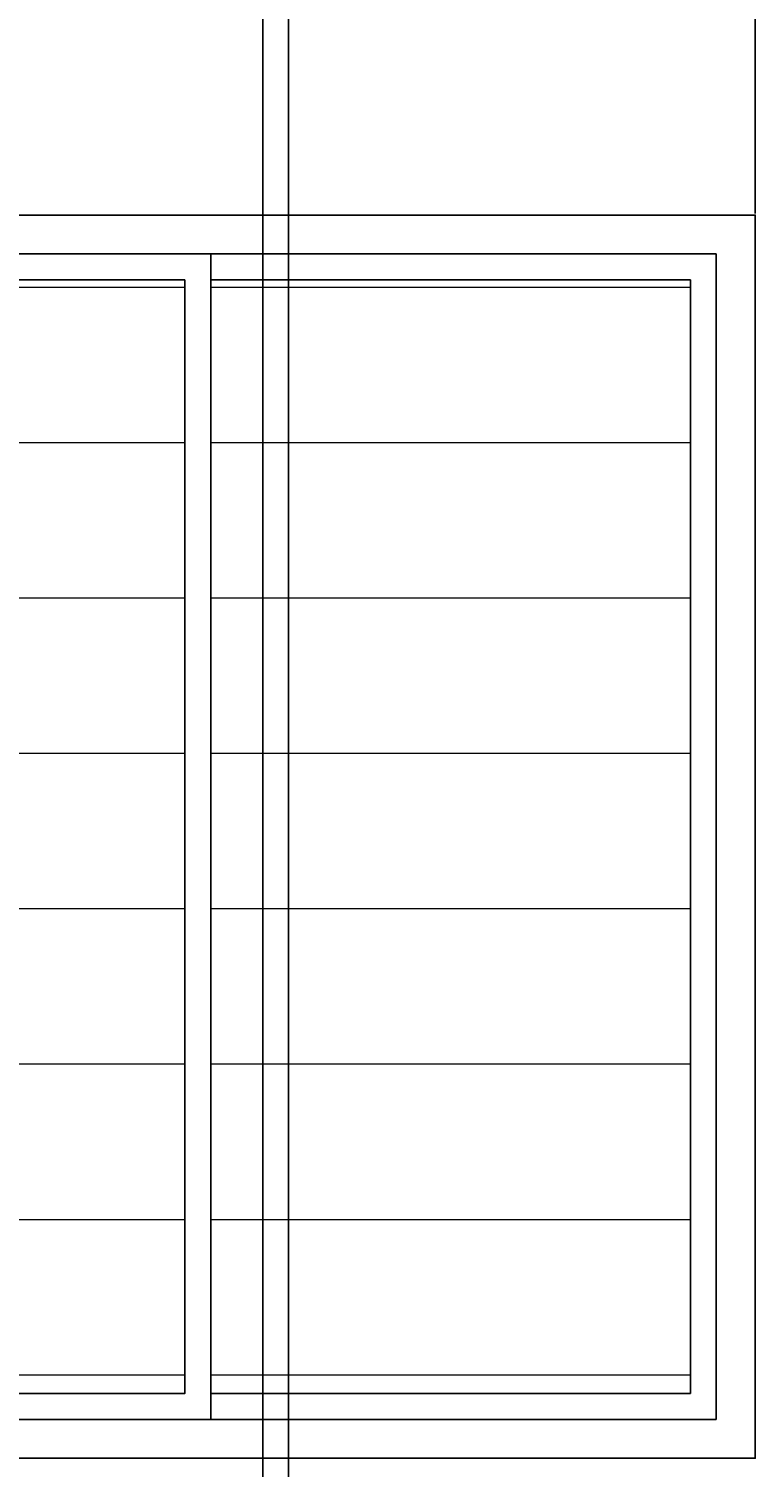
# Model space of a CAD drawing. Units: inches. Extents: x -6 to 289, y -8 to 323.
# Tile 38 of 107: x 202 to 230, y 68 to 124. Entities that reach past the tile are written whole.
import ezdxf

# ---------------------------------------------------------------- set-up
doc = ezdxf.new("R2010")
doc.units = ezdxf.units.IN
doc.header["$MEASUREMENT"] = 0
for name, color, linetype, lineweight in [('A-ANNO-DIMS', 2, 'Continuous', 18), ('A-ELEV-PATT', 8, 'Continuous', 13), ('A-GLAZ', 4, 'Continuous', 25)]:
    doc.layers.add(name, color=color, linetype=linetype, lineweight=lineweight)
doc.styles.get("Standard").update_dxf_attribs({"font": 'arial.ttf'})
doc.dimstyles.get("Standard").update_dxf_attribs({"dimtxt": 0.18, "dimasz": 0.18, "dimexe": 0.18, "dimexo": 0.0625, "dimgap": 0.09, "dimtad": 0, "dimtih": 1, "dimtoh": 1, "dimdec": 4, "dimzin": 0, "dimdsep": 46, "dimtxsty": 'Standard', "dimcen": 0.09, "dimadec": 0, "dimazin": 0, "dimtfac": 1, "dimtdec": 4, "dimtofl": 0, "dimtmove": 0, "dimatfit": 3, "dimfxl": 1, "dimtolj": 1, "dimtzin": 0, "dimarcsym": 0})

# ---------------------------------------------------------------- blocks, each defined once
blk = doc.blocks.new('*U4')
for p, q in [((1.5, 1.5), (1.5, 46.5)), ((1.5, 46.5), (21, 46.5)), ((21, 1.5), (21, 46.5)), ((21, 46.5), (40.5, 46.5)), ((40.5, 46.5), (40.5, 1.5)), ((21, 1.5), (1.5, 1.5)), ((40.5, 1.5), (21, 1.5))]:
    blk.add_line(p, q)
blk.add_lwpolyline([(0, 0), (0, 48), (42, 48), (42, 0)], close=True)
for points in [[(20, 45.5), (20, 2.5), (2.5, 2.5), (2.5, 45.5), (20, 45.5)], [(21, 45.5), (39.5, 45.5), (39.5, 2.5), (21, 2.5)]]:
    blk.add_lwpolyline(points)
blk = doc.blocks.new('*D42')
at = {"layer": 'A-ANNO-DIMS', "color": 0, "lineweight": -2, "transparency": 16777216}
for p, q in [((190.792, 224.326), (190.792, -8.391)), ((211.292, 224.326), (211.292, -8.391)), ((190.972, -8.211), (200.716, -8.211)), ((211.112, -8.211), (201.368, -8.211))]:
    blk.add_line(p, q, dxfattribs=at)
at = {"layer": 'A-ANNO-DIMS', "color": 0, "transparency": 16777216}
for points in [[(190.972, -8.181), (190.972, -8.241), (190.792, -8.211)], [(211.112, -8.181), (211.112, -8.241), (211.292, -8.211)]]:
    blk.add_solid(points, dxfattribs=at)
at = {"layer": 'Defpoints', "color": 0, "transparency": 16777216}
for p in [(190.792, 224.389), (211.292, 224.389), (211.292, -8.211)]:
    blk.add_point(p, dxfattribs=at)
at = {"layer": 'A-ANNO-DIMS', "color": 0, "transparency": 16777216, "insert": (201.042, -8.211), "char_height": 0.18, "attachment_point": 5}
blk.add_mtext('\\A1;20.5', dxfattribs=at)
blk = doc.blocks.new('*D43')
at = {"layer": 'A-ANNO-DIMS', "color": 0, "lineweight": -2, "transparency": 16777216}
for p, q in [((211.292, 224.326), (211.292, -8.391)), ((212.292, 224.326), (212.292, -8.391)), ((211.472, -8.211), (211.669, -8.211)), ((212.112, -8.211), (211.915, -8.211))]:
    blk.add_line(p, q, dxfattribs=at)
at = {"layer": 'A-ANNO-DIMS', "color": 0, "transparency": 16777216}
for points in [[(211.472, -8.181), (211.472, -8.241), (211.292, -8.211)], [(212.112, -8.181), (212.112, -8.241), (212.292, -8.211)]]:
    blk.add_solid(points, dxfattribs=at)
at = {"layer": 'Defpoints', "color": 0, "transparency": 16777216}
for p in [(211.292, 224.389), (212.292, 224.389), (212.292, -8.211)]:
    blk.add_point(p, dxfattribs=at)
at = {"layer": 'A-ANNO-DIMS', "color": 0, "transparency": 16777216, "insert": (211.792, -8.211), "char_height": 0.18, "attachment_point": 5}
blk.add_mtext('\\A1;1', dxfattribs=at)
blk = doc.blocks.new('*D44')
at = {"layer": 'A-ANNO-DIMS', "color": 0, "lineweight": -2, "transparency": 16777216}
for p, q in [((212.292, 224.326), (212.292, -8.391)), ((233.792, 224.326), (233.792, -8.391)), ((212.472, -8.211), (222.716, -8.211)), ((233.612, -8.211), (223.368, -8.211))]:
    blk.add_line(p, q, dxfattribs=at)
at = {"layer": 'A-ANNO-DIMS', "color": 0, "transparency": 16777216}
for points in [[(212.472, -8.181), (212.472, -8.241), (212.292, -8.211)], [(233.612, -8.181), (233.612, -8.241), (233.792, -8.211)]]:
    blk.add_solid(points, dxfattribs=at)
at = {"layer": 'Defpoints', "color": 0, "transparency": 16777216}
for p in [(212.292, 224.389), (233.792, 224.389), (233.792, -8.211)]:
    blk.add_point(p, dxfattribs=at)
at = {"layer": 'A-ANNO-DIMS', "color": 0, "transparency": 16777216, "insert": (223.042, -8.211), "char_height": 0.18, "attachment_point": 5}
blk.add_mtext('\\A1;21.5', dxfattribs=at)
blk = doc.blocks.new('*D80')
at = {"layer": 'A-ANNO-DIMS', "color": 0, "lineweight": -2, "transparency": 16777216}
for p, q in [((188.292, 116.842), (188.292, 322.969)), ((188.472, 322.789), (209.07, 322.789)), ((230.112, 322.789), (209.513, 322.789)), ((230.292, 116.842), (230.292, 322.969))]:
    blk.add_line(p, q, dxfattribs=at)
at = {"layer": 'A-ANNO-DIMS', "color": 0, "transparency": 16777216}
for points in [[(188.472, 322.819), (188.472, 322.759), (188.292, 322.789)], [(230.112, 322.819), (230.112, 322.759), (230.292, 322.789)]]:
    blk.add_solid(points, dxfattribs=at)
at = {"layer": 'Defpoints', "color": 0, "transparency": 16777216}
for p in [(230.292, 322.789), (188.292, 116.779), (230.292, 116.779)]:
    blk.add_point(p, dxfattribs=at)
at = {"layer": 'A-ANNO-DIMS', "color": 0, "transparency": 16777216, "insert": (209.292, 322.789), "char_height": 0.18, "attachment_point": 5}
blk.add_mtext('\\A1;42', dxfattribs=at)

msp = doc.modelspace()

# ---------------------------------------------------------------- hatches: boundary and pattern name
at = {"layer": 'A-ELEV-PATT'}
h = msp.add_hatch(dxfattribs=at)
h.set_pattern_fill('_USER', color=256, scale=6, pattern_type=0)
h.set_pattern_definition([(0, (0, 0), (0, 6), [])])
h.paths.add_polyline_path([(184.1244, 48.0851), (124.008, 48.0851), (124.008, 10.2888), (184.1244, 10.2888)])
h.paths.add_polyline_path([(244.2408, 48.0851), (186.3604, 48.0851), (186.3604, 10.2888), (244.2408, 10.2888)])
h.paths.add_polyline_path([(208.2918, 114.2795), (190.7918, 114.2795), (190.7918, 71.2795), (208.2918, 71.2795)])
h.paths.add_polyline_path([(227.7918, 114.2795), (209.2918, 114.2795), (209.2918, 71.2795), (227.7918, 71.2795)])
h.paths.add_polyline_path([(211.2918, 224.3887), (190.7918, 224.3887), (190.7918, 162.3484), (211.2918, 162.3484)])
h.paths.add_polyline_path([(233.7918, 224.3887), (212.2918, 224.3887), (212.2918, 162.3484), (233.7918, 162.3484)])
h.paths.add_polyline_path([(166.3835, 224.154), (147.8835, 224.154), (147.8835, 181.154), (166.3835, 181.154)])
h.paths.add_polyline_path([(146.8835, 224.154), (129.3835, 224.154), (129.3835, 181.154), (146.8835, 181.154)])

# ---------------------------------------------------------------- block references
at = {"layer": 'A-GLAZ'}
msp.add_blockref('*U4', (188.2918, 68.7795), dxfattribs=at)

# ---------------------------------------------------------------- dimensions: what is measured, and where the dimension line sits
at = {"layer": 'A-ANNO-DIMS'}
for base, p1, p2, override, picture, middle in [((230.2918, 322.7888), (188.2918, 116.7795), (230.2918, 116.7795), {"dimdec": 0, "dimlfac": 1, "dimrnd": 0, "dimzin": 0, "dimdsep": 46, "dimlunit": 2}, '*D80', (209.2918, 322.7888)), ((211.2918, -8.2112), (190.7918, 224.3887), (211.2918, 224.3887), {"dimdec": 1, "dimlfac": 1, "dimrnd": 0, "dimzin": 0, "dimdsep": 46, "dimlunit": 2}, '*D42', (201.0418, -8.2112)), ((212.2918, -8.2112), (211.2918, 224.3887), (212.2918, 224.3887), {"dimdec": 0, "dimlfac": 1, "dimrnd": 0, "dimzin": 0, "dimdsep": 46, "dimlunit": 2}, '*D43', (211.7918, -8.2112)), ((233.7918, -8.2112), (212.2918, 224.3887), (233.7918, 224.3887), {"dimdec": 1, "dimlfac": 1, "dimrnd": 0, "dimzin": 0, "dimdsep": 46, "dimlunit": 2}, '*D44', (223.0418, -8.2112))]:
    dim = msp.add_linear_dim(base=base, p1=p1, p2=p2, dimstyle='Standard', override=override, dxfattribs=at)
    dim.commit()
    dim.dimension.update_dxf_attribs({"geometry": picture, "text_midpoint": middle})

doc.saveas('drawing.dxf')
